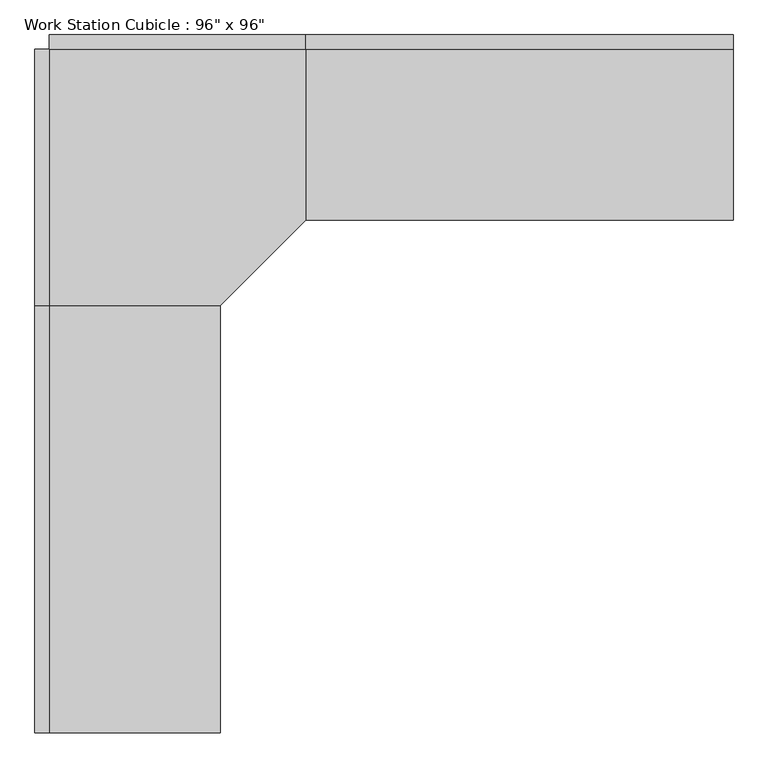
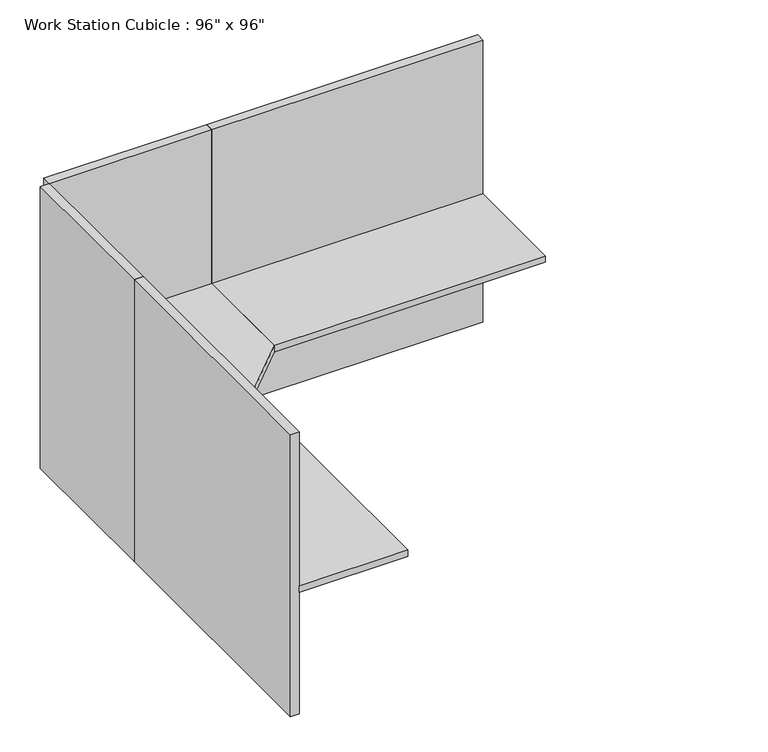
"""IFC4 building model written with IfcOpenShell, lengths in millimetres: furniture geometry."""

from ifc_helpers import new_model, si_unit, frame, origin, origin_with_axes, place, context, project, spatial, polyline, outline, extrude, source, transform, mapped, element, save


def furniture_45e3acac(model_context):
    return source(origin(), model_context, "Body", "SweptSolid", [
        extrude(outline(polyline([(-80.9317522, -545.8230076), (833.4682478, -545.8230076), (833.4682478, -1155.4230076), (528.6682478, -1460.2230076), (-80.9317522, -1460.2230076), (-80.9317522, -545.8230076)])), frame((0.0, 0.0, 723.9), z_axis=(0.0, 0.0, 1.0), x_axis=(1.0, 0.0, 0.0)), (0.0, 0.0, 1.0), 38.1),
        extrude(outline(polyline([(528.6682478, -2984.2230076), (-80.9317522, -2984.2230076), (-80.9317522, -1460.2230076), (528.6682478, -1460.2230076), (528.6682478, -2984.2230076)])), frame((0.0, 0.0, 723.9), z_axis=(0.0, 0.0, 1.0), x_axis=(1.0, 0.0, 0.0)), (0.0, 0.0, 1.0), 38.1),
        extrude(outline(polyline([(2357.4682478, -1155.4230076), (833.4682478, -1155.4230076), (833.4682478, -545.8230076), (2357.4682478, -545.8230076), (2357.4682478, -1155.4230076)])), frame((0.0, 0.0, 723.9), z_axis=(0.0, 0.0, 1.0), x_axis=(1.0, 0.0, 0.0)), (0.0, 0.0, 1.0), 38.1),
        extrude(outline(polyline([(2357.4682478, -545.8230076), (833.4682478, -545.8230076), (833.4682478, -495.0230076), (2357.4682478, -495.0230076), (2357.4682478, -545.8230076)])), origin_with_axes(), (0.0, 0.0, 1.0), 1676.4),
        extrude(outline(polyline([(833.4682478, -545.8230076), (-80.9317522, -545.8230076), (-80.9317522, -495.0230076), (833.4682478, -495.0230076), (833.4682478, -545.8230076)])), origin_with_axes(), (0.0, 0.0, 1.0), 1676.4),
        extrude(outline(polyline([(-80.9317522, -1460.2230076), (-131.7317522, -1460.2230076), (-131.7317522, -545.8230076), (-80.9317522, -545.8230076), (-80.9317522, -1460.2230076)])), origin_with_axes(), (0.0, 0.0, 1.0), 1676.4),
        extrude(outline(polyline([(-80.9317522, -2984.2230076), (-131.7317522, -2984.2230076), (-131.7317522, -1460.2230076), (-80.9317522, -1460.2230076), (-80.9317522, -2984.2230076)])), origin_with_axes(), (0.0, 0.0, 1.0), 1676.4),
    ])


if __name__ == "__main__":
    model = new_model("IFC4")
    model_context = context("Model", 3, world=origin())
    ifc_project = project(units=[si_unit("LENGTHUNIT", "METRE", prefix="MILLI")], contexts=[model_context])
    site = spatial("IfcSite", under=ifc_project)
    building = spatial("IfcBuilding", under=site)
    placement = place(None, origin())
    furniture_shape = furniture_45e3acac(model_context)
    element("IfcFurniture", 1, ObjectType="Work Station Cubicle : 96\" x 96\"", at=placement, inside=building, context=model_context, shape_type="MappedRepresentation", body=[
        mapped(furniture_shape, transform((0.0, 0.0, 0.0), x_axis=(1.0, 0.0, 0.0), y_axis=(0.0, 1.0, 0.0), z_axis=(0.0, 0.0, 1.0))),
    ])
    save(model, "model.ifc")

# Revit data of these elements
# Type "Work Station Cubicle : 96\" x 96\""
#   Assembly Code = "E2020"
#   Desktop Height = 2' - 6"
#   Desktop1 Width = 2' - 0"
#   Desktop2 Width = 2' - 0"
#   Panel Height = 5' - 6"
#   Panel1 Length = 5' - 0"
#   Panel2 Length = 5' - 0"
#   Cube Panel Material = Textile - Light Gray
#   Work Top Material = Laminate, Ivory, Matte
# Element 1 (IfcFurniture, "Work Station Cubicle : 96\" x 96\"")
#   Materials on its faces: "Textile - Light Gray", "Laminate, Ivory, Matte"
# Materials
#   "Textile - Light Gray": class "Fabric", colour RGB 204 204 204, transparency 0
#   "Laminate, Ivory, Matte": class "Plastic", colour RGB 247 247 239, transparency 0, Description = "Plastic Laminate - Ivory, Matte", Cost = 0
